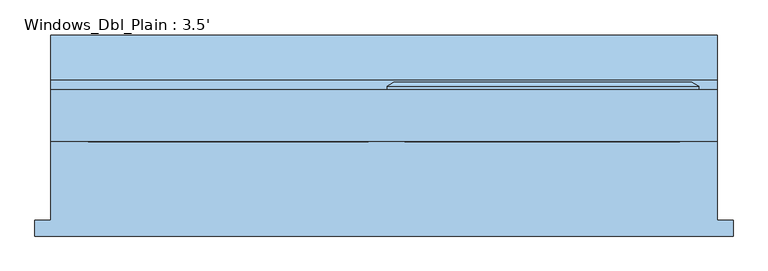
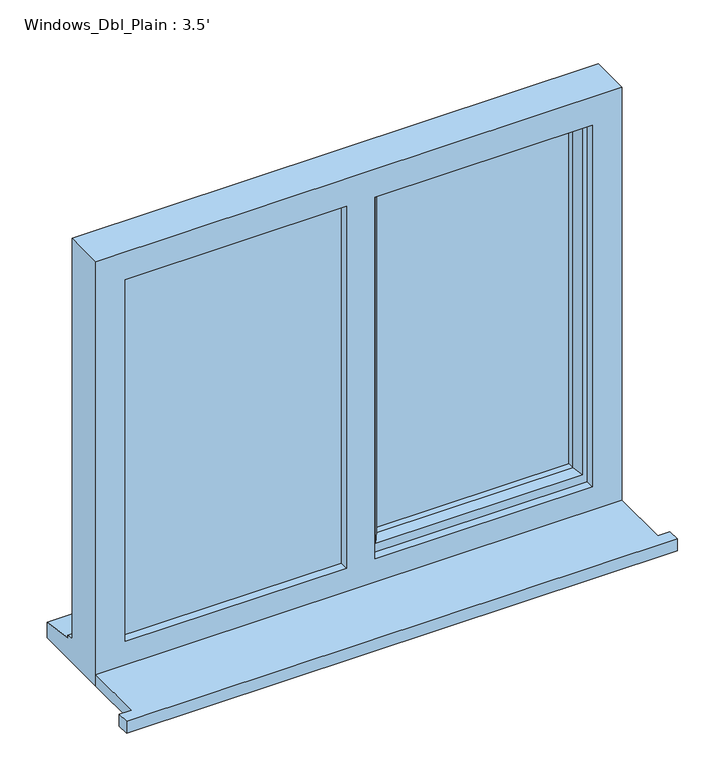
"""IFC4 building model written with IfcOpenShell, lengths in millimetres: window geometry, Windows_Dbl_Plain : 3.5'."""

from ifc_helpers import new_model, si_unit, frame, origin, place, context, project, spatial, polyline, outline, extrude, faceted_brep, source, transform, mapped, element, save


def windows_dbl_plain_3_5_9bb0dad6(model_context):
    return source(origin(), model_context, "Body", "SolidModel", [
        extrude(outline(polyline([(-843.4, -146.0834322), (-843.4, -121.0834322), (-818.4, -121.0834322), (-818.4, 4.9965678), (248.4, 4.9965678), (248.4, -121.0834322), (273.4, -121.0834322), (273.4, -146.0834322), (-843.4, -146.0834322)])), frame((0.0, 0.0, 1200.0), z_axis=(0.0, 0.0, 1.0), x_axis=(1.0, 0.0, 0.0)), (0.0, 0.0, 1.0), 25.0),
        faceted_brep([(-280.0, 87.9965678, 2080.0), (-280.0, 93.7700705, 2080.0), (-280.0, 93.7700705, 1253.0), (-280.0, 87.9965678, 1253.0), (-270.0, 22.9965678, 2070.0), (-270.0, 87.9965678, 2070.0), (-270.0, 87.9965678, 1263.0), (-270.0, 22.9965678, 1263.0), (-230.0, 37.4894677, 2030.0), (-240.1480377, 22.9965678, 2040.1480377), (-240.1480377, 22.9965678, 1292.8519623), (-230.0, 37.4894677, 1303.0), (-230.0, 51.9965678, 2030.0), (-230.0, 51.9965678, 1303.0), (-240.0, 75.9965678, 2040.0), (-240.0, 51.9965678, 2040.0), (-240.0, 51.9965678, 1293.0), (-240.0, 75.9965678, 1293.0), (-230.0, 93.7700705, 2030.0), (-230.0, 75.9965678, 2030.0), (-230.0, 75.9965678, 1303.0), (-230.0, 93.7700705, 1303.0), (-247.4457548, 99.5435732, 2047.4457548), (-247.4457548, 99.5435732, 1285.5542452), (-269.2153903, 99.5435732, 2069.2153903), (-269.2153903, 99.5435732, 1263.7846097), (218.4, 93.7700705, 1253.0), (218.4, 87.9965678, 1253.0), (208.4, 87.9965678, 1263.0), (208.4, 22.9965678, 1263.0), (178.5480377, 22.9965678, 1292.8519623), (168.4, 37.4894677, 1303.0), (168.4, 51.9965678, 1303.0), (178.4, 51.9965678, 1293.0), (178.4, 75.9965678, 1293.0), (168.4, 75.9965678, 1303.0), (168.4, 93.7700705, 1303.0), (185.8457548, 99.5435732, 1285.5542452), (207.6153903, 99.5435732, 1263.7846097), (218.4, 93.7700705, 2080.0), (218.4, 87.9965678, 2080.0), (208.4, 87.9965678, 2070.0), (208.4, 22.9965678, 2070.0), (178.5480377, 22.9965678, 2040.1480377), (168.4, 37.4894677, 2030.0), (168.4, 51.9965678, 2030.0), (178.4, 51.9965678, 2040.0), (178.4, 75.9965678, 2040.0), (168.4, 75.9965678, 2030.0), (168.4, 93.7700705, 2030.0), (185.8457548, 99.5435732, 2047.4457548), (207.6153903, 99.5435732, 2069.2153903)], [[[0, 1, 2, 3]], [[4, 5, 6, 7]], [[8, 9, 10, 11]], [[12, 8, 11, 13]], [[14, 15, 16, 17]], [[18, 19, 20, 21]], [[22, 18, 21, 23]], [[1, 24, 25, 2]], [[3, 2, 26, 27]], [[7, 6, 28, 29]], [[11, 10, 30, 31]], [[13, 11, 31, 32]], [[17, 16, 33, 34]], [[21, 20, 35, 36]], [[23, 21, 36, 37]], [[2, 25, 38, 26]], [[27, 26, 39, 40]], [[29, 28, 41, 42]], [[31, 30, 43, 44]], [[32, 31, 44, 45]], [[34, 33, 46, 47]], [[36, 35, 48, 49]], [[37, 36, 49, 50]], [[26, 38, 51, 39]], [[40, 39, 1, 0]], [[3, 27, 40, 0], [5, 41, 28, 6]], [[42, 41, 5, 4]], [[7, 29, 42, 4], [9, 43, 30, 10]], [[44, 43, 9, 8]], [[45, 44, 8, 12]], [[15, 46, 33, 16], [13, 32, 45, 12]], [[47, 46, 15, 14]], [[17, 34, 47, 14], [19, 48, 35, 20]], [[49, 48, 19, 18]], [[50, 49, 18, 22]], [[24, 51, 38, 25], [23, 37, 50, 22]], [[39, 51, 24, 1]]]),
        extrude(outline(polyline([(2050.0, -310.0), (2070.0, -310.0), (2070.0, -778.4), (1263.0, -778.4), (1263.0, -310.0), (1283.0, -310.0), (1283.0, -758.4), (2050.0, -758.4), (2050.0, -310.0)])), frame((0.0, 46.9965678, 0.0), z_axis=(0.0, 1.0, 0.0), x_axis=(0.0, 0.0, 1.0)), (0.0, 0.0, 1.0), 41.0),
        faceted_brep([(248.4, 4.9965678, 2110.0), (-818.4, 4.9965678, 2110.0), (-818.4, 4.9965678, 1200.0), (248.4, 4.9965678, 1200.0), (188.4, 4.9965678, 2050.0), (188.4, 4.9965678, 1275.0), (-252.0, 4.9965678, 1275.0), (-252.0, 4.9965678, 2050.0), (-310.0, 4.9965678, 2050.0), (-310.0, 4.9965678, 1275.0), (-758.4, 4.9965678, 1275.0), (-758.4, 4.9965678, 2050.0), (-818.4, 87.9965678, 2110.0), (-818.4, 87.9965678, 1251.0), (-818.4, 102.9965678, 1249.68767), (-818.4, 102.9965678, 1244.7449676), (-818.4, 175.4965678, 1233.8088847), (-818.4, 175.4965678, 1200.0), (248.4, 87.9965678, 2110.0), (248.4, 87.9965678, 1251.0), (-778.4, 87.9965678, 2070.0), (-778.4, 87.9965678, 1263.0), (-310.0, 87.9965678, 1263.0), (-310.0, 87.9965678, 2070.0), (-270.0, 87.9965678, 2070.0), (-270.0, 87.9965678, 1263.0), (208.4, 87.9965678, 1263.0), (208.4, 87.9965678, 2070.0), (-778.4, 22.9965678, 2070.0), (-778.4, 22.9965678, 1263.0), (-300.0, 22.9965678, 2070.0), (-300.0, 22.9965678, 1263.0), (-310.0, 22.9965678, 2050.0), (-758.4, 22.9965678, 2050.0), (-758.4, 22.9965678, 1275.0), (-310.0, 22.9965678, 1275.0), (-270.0, 22.9965678, 2070.0), (208.4, 22.9965678, 2070.0), (208.4, 22.9965678, 1263.0), (-270.0, 22.9965678, 1263.0), (188.4, 22.9965678, 2050.0), (-252.0, 22.9965678, 2050.0), (-252.0, 22.9965678, 1275.0), (188.4, 22.9965678, 1275.0), (-310.0, 46.9965678, 2070.0), (-300.0, 46.9965678, 2070.0), (248.4, 175.4965678, 1200.0), (248.4, 175.4965678, 1233.8088847), (248.4, 102.9965678, 1244.7449676), (248.4, 102.9965678, 1249.68767), (-300.0, 46.9965678, 1263.0), (-310.0, 46.9965678, 1263.0)], [[[0, 1, 2, 3], [4, 5, 6, 7], [8, 9, 10, 11]], [[2, 1, 12, 13, 14, 15, 16, 17]], [[13, 12, 18, 19], [20, 21, 22, 23], [24, 25, 26, 27]], [[21, 20, 28, 29]], [[28, 30, 31, 29], [32, 33, 34, 35]], [[36, 37, 38, 39], [40, 41, 42, 43]], [[33, 11, 10, 34]], [[1, 0, 18, 12]], [[28, 20, 23, 44, 45, 30]], [[27, 37, 36, 24]], [[11, 33, 32, 8]], [[40, 4, 7, 41]], [[19, 18, 0, 3, 46, 47, 48, 49]], [[27, 26, 38, 37]], [[4, 40, 43, 5]], [[45, 50, 31, 30]], [[50, 45, 44, 51]], [[51, 44, 23, 22]], [[25, 24, 36, 39]], [[41, 7, 6, 42]], [[8, 32, 35, 9]], [[46, 3, 2, 17]], [[47, 46, 17, 16]], [[48, 47, 16, 15]], [[49, 48, 15, 14]], [[19, 49, 14, 13]], [[22, 21, 29, 31, 50, 51]], [[26, 25, 39, 38]], [[6, 5, 43, 42]], [[35, 34, 10, 9]]]),
        extrude(outline(polyline([(-778.4, 46.9965678), (-300.0, 46.9965678), (-300.0, 22.9965678), (-778.4, 22.9965678), (-778.4, 46.9965678)])), frame((0.0, 0.0, 1263.0), z_axis=(0.0, 0.0, 1.0), x_axis=(1.0, 0.0, 0.0)), (0.0, 0.0, 1.0), 807.0),
        extrude(outline(polyline([(178.4, 51.9965678), (-240.0, 51.9965678), (-240.0, 75.9965678), (178.4, 75.9965678), (178.4, 51.9965678)])), frame((0.0, 0.0, 1293.0), z_axis=(0.0, 0.0, 1.0), x_axis=(1.0, 0.0, 0.0)), (0.0, 0.0, 1.0), 747.0),
    ])


if __name__ == "__main__":
    model = new_model("IFC4")
    model_context = context("Model", 3, world=origin())
    ifc_project = project(units=[si_unit("LENGTHUNIT", "METRE", prefix="MILLI")], contexts=[model_context])
    site = spatial("IfcSite", under=ifc_project)
    building = spatial("IfcBuilding", under=site)
    placement = place(None, origin())
    windows_dbl_plain_3_5_shape = windows_dbl_plain_3_5_9bb0dad6(model_context)
    element("IfcWindow", 1, ObjectType="Windows_Dbl_Plain : 3.5'", at=placement, inside=building, context=model_context, shape_type="MappedRepresentation", body=[
        mapped(windows_dbl_plain_3_5_shape, transform((0.0, 0.0, 0.0), x_axis=(1.0, 0.0, 0.0), y_axis=(0.0, 1.0, 0.0), z_axis=(0.0, 0.0, 1.0))),
    ])
    save(model, "model.ifc")

# Revit data of these elements
# Type "Windows_Dbl_Plain : 3.5'"
#   Type Mark = "64"
#   Operation = "DoublePanelVertical"
#   Construction Type Id = "GSP4R"
#   Manufacturer = "Revit"
#   Keynote = "L10"
#   Analytic Construction = "1/8 in Pilkington single glazing"
#   Wrap Layers (Ext) from Ext = 102.5 mm
#   Wrap Layers (Int) from Ext = 177.5 mm
#   Window Board Projection = 25 mm
#   Window Board Extension = 25 mm
#   Visual Light Transmittance = 0.9
#   Solar Heat Gain Coefficient = 0.78
#   Rough Width = 1066.8 mm
#   Rough Height = 910 mm
#   Height = 910 mm
#   Width = 1066.8 mm
#   Heat Transfer Coefficient (U) = 3.6886 W/(m²·K)
#   Glazing Thickness = 24 mm
#   FrameOffset - External = 50 mm
#   Frame Depth = 65 mm
#   Default Head Height = 2110 mm
#   Cill Depth = 87.5 mm
#   Cavity Closer Width = 50 mm
#   Cavity Closer Offset from Ext = 102.5 mm
#   Cavity Closer Depth = 85 mm
#   Vis - Cavity Closers = yes
#   Define Thermal Properties by = 1
#   Material Trim = Window Frame
#   Material Glass = Glass
#   Material Frame = Window Frame
#   Wall Closure = (empty or 0)
# Element 1 (IfcWindow, "Windows_Dbl_Plain : 3.5'")
#   Materials on its faces: "Window Frame", "Glass"
# Materials
#   "Window Frame": colour RGB 249 249 249, transparency 0, Keynote = "L10", Cost = 0
#   "Glass": class "Glass", colour RGB 0 128 192, transparency 0.9, Description = "Soda Lime Glass", Cost = 0
